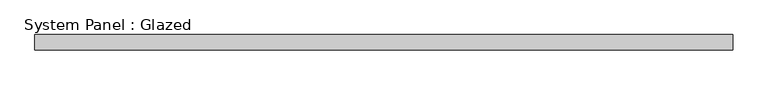
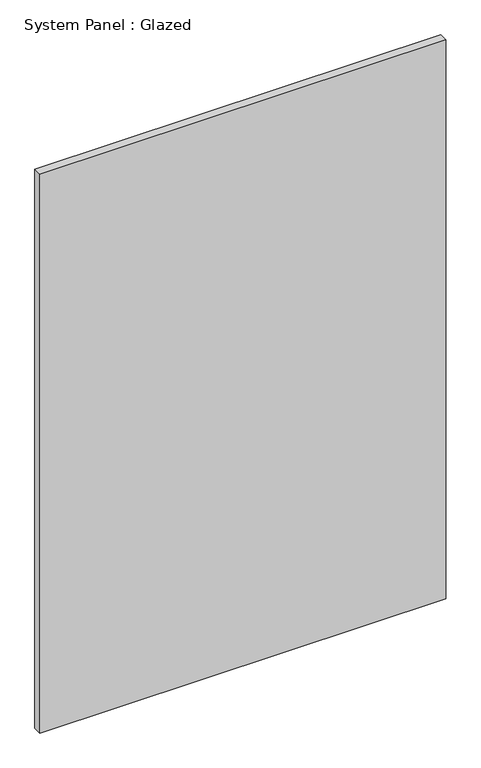
"""IFC4 building model written with IfcOpenShell, lengths in millimetres: plate geometry, System Panel : Glazed."""

from ifc_helpers import new_model, si_unit, origin, origin_with_axes, place, context, project, spatial, polyline, outline, extrude, source, transform, mapped, element, save


def system_panel_glazed_1700d241(model_context):
    return source(origin(), model_context, "Body", "SweptSolid", [
        extrude(outline(polyline([(584.2, 19.05), (-584.2, 19.05), (-584.2, 44.45), (584.2, 44.45), (584.2, 19.05)])), origin_with_axes(), (0.0, 0.0, 1.0), 1701.8),
    ])


if __name__ == "__main__":
    model = new_model("IFC4")
    model_context = context("Model", 3, world=origin())
    ifc_project = project(units=[si_unit("LENGTHUNIT", "METRE", prefix="MILLI")], contexts=[model_context])
    site = spatial("IfcSite", under=ifc_project)
    building = spatial("IfcBuilding", under=site)
    placement = place(None, origin())
    system_panel_glazed_shape = system_panel_glazed_1700d241(model_context)
    element("IfcPlate", 1, ObjectType="System Panel : Glazed", at=placement, inside=building, context=model_context, shape_type="MappedRepresentation", body=[
        mapped(system_panel_glazed_shape, transform((0.0, 0.0, 0.0), x_axis=(1.0, 0.0, 0.0), y_axis=(0.0, 1.0, 0.0), z_axis=(0.0, 0.0, 1.0))),
    ])
    save(model, "model.ifc")

# Revit data of these elements
# Type "System Panel : Glazed"
#   Construction Type Id = "GSP4R"
#   Analytic Construction = "1/8 in Pilkington single glazing"
#   Visual Light Transmittance = 0.9
#   Solar Heat Gain Coefficient = 0.86
#   Heat Transfer Coefficient (U) = 1.18115 BTU/(h·ft²·°F)
# Element 1 (IfcPlate, "System Panel : Glazed")
#   Materials on its faces: "Glass"
# Materials
#   "Glass": class "Glass", colour RGB 0 128 192, transparency 0.75, Description = "Soda Lime Glass", Cost = 0
